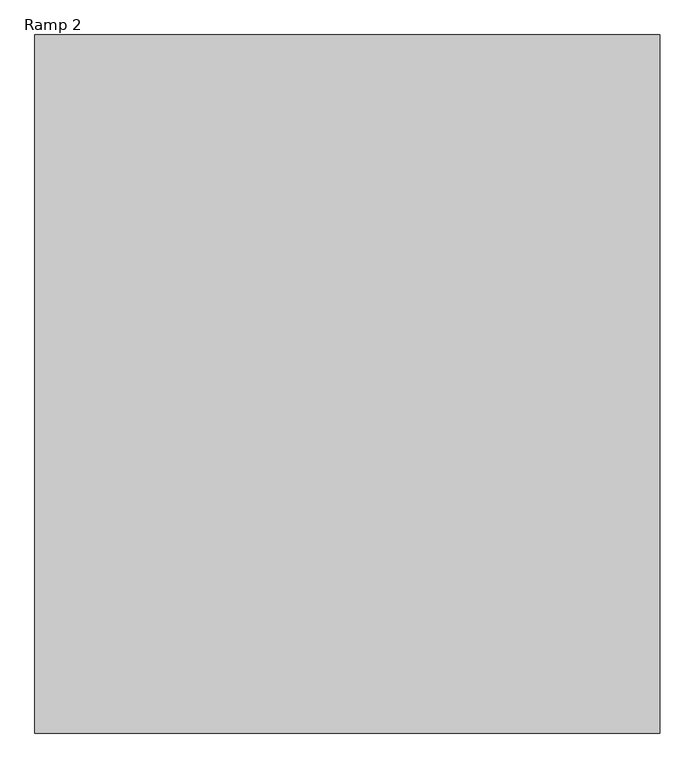
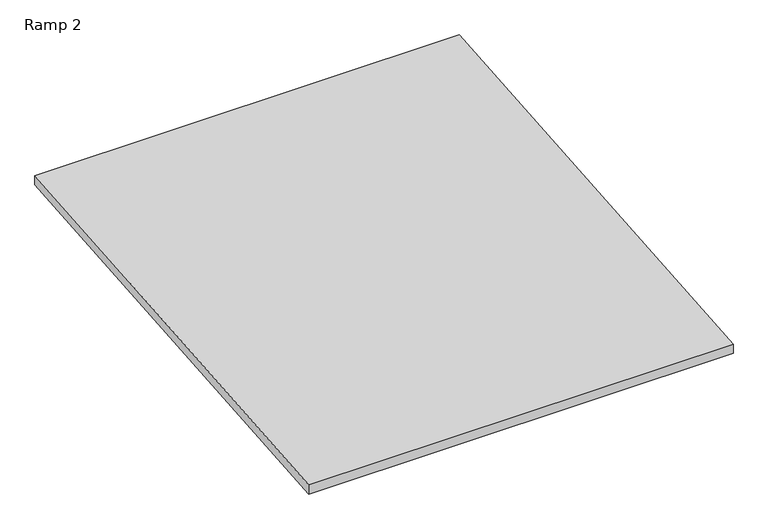
"""IFC4 building model written with IfcOpenShell, lengths in millimetres: ramp geometry, Ramp 2."""

from ifc_helpers import new_model, si_unit, frame, origin, place, context, project, spatial, polyline, outline, extrude, source, transform, mapped, element, save


def ramp_2_4435543f(model_context):
    return source(origin(), model_context, "Body", "SweptSolid", [
        extrude(outline(polyline([(-363.1028667, -304.8), (3294.4971333, 0.0), (3294.4971333, -76.4641256), (-363.1028667, -381.2641256), (-363.1028667, -304.8)])), frame((23094.6569618, 0.0, 0.0), z_axis=(1.0, 0.0, 0.0), x_axis=(0.0, 1.0, 0.0)), (0.0, 0.0, 1.0), 3276.6),
    ])


if __name__ == "__main__":
    model = new_model("IFC4")
    model_context = context("Model", 3, world=origin())
    ifc_project = project(units=[si_unit("LENGTHUNIT", "METRE", prefix="MILLI")], contexts=[model_context])
    site = spatial("IfcSite", under=ifc_project)
    building = spatial("IfcBuilding", under=site)
    placement = place(None, origin())
    ramp_2_shape = ramp_2_4435543f(model_context)
    element("IfcRamp", 1, ObjectType="Ramp 2", at=placement, inside=building, context=model_context, shape_type="MappedRepresentation", body=[
        mapped(ramp_2_shape, transform((0.0, 0.0, 0.0), x_axis=(1.0, 0.0, 0.0), y_axis=(0.0, 1.0, 0.0), z_axis=(0.0, 0.0, 1.0))),
    ])
    save(model, "model.ifc")
